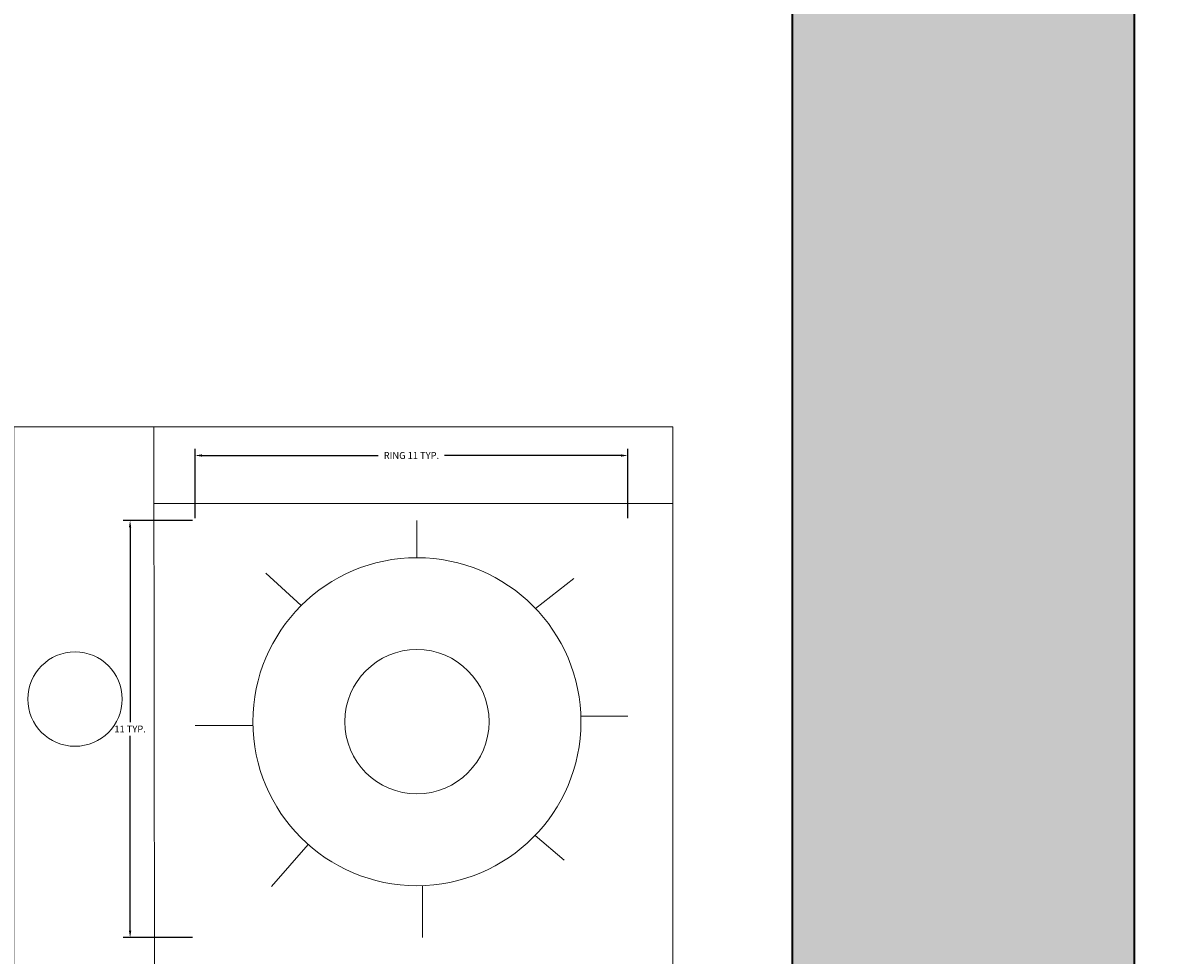
# Model space of a CAD drawing. Units: inches. Extents: x 1568 to 2529, y 2149 to 2897.
# Tile 7 of 16: x 1944 to 1974, y 2386 to 2410. Entities that reach past the tile are written whole.
import ezdxf

# ---------------------------------------------------------------- set-up
doc = ezdxf.new("R2010")
doc.units = ezdxf.units.IN
for name, color, linetype, lineweight in [('A-ANNO-DIMS', 2, 'Continuous', 18), ('A-EQPM', 8, 'Continuous', 18), ('A-WALL-PATT', 172, 'Continuous', 13), ('wall', 7, 'Continuous', 35)]:
    doc.layers.add(name, color=color, linetype=linetype, lineweight=lineweight)
doc.styles.get("Standard").update_dxf_attribs({"font": 'arial.ttf'})
doc.dimstyles.get("Standard").update_dxf_attribs({"dimtxt": 0.18, "dimasz": 0.18, "dimexe": 0.18, "dimexo": 0.0625, "dimgap": 0.09, "dimtad": 0, "dimtih": 1, "dimtoh": 1, "dimdec": 4, "dimzin": 0, "dimdsep": 46, "dimtxsty": 'Standard', "dimcen": 0.09, "dimadec": 0, "dimazin": 0, "dimtfac": 1, "dimtdec": 4, "dimtofl": 0, "dimtmove": 0, "dimatfit": 3, "dimfxl": 1, "dimtolj": 1, "dimtzin": 0, "dimarcsym": 0})

# ---------------------------------------------------------------- blocks, each defined once
blk = doc.blocks.new('COOKTOP-BURNER')
for p, q in [((0.001, 4.315), (0.001, 5.296)), ((-3.048, 3.054), (-3.977, 3.91)), ((3.12, 2.981), (4.125, 3.765)), ((4.312, 0.148), (5.549, 0.148)), ((-4.314, -0.098), (-5.839, -0.098)), ((3.11, -2.99), (3.87, -3.639)), ((-2.86, -3.23), (-3.831, -4.332)), ((0.143, -4.312), (0.143, -5.681))]:
    blk.add_line(p, q)
for radius in [4.315, 1.899]:
    blk.add_circle((0, 0), radius)
blk = doc.blocks.new('*D25')
at = {"layer": 'A-ANNO-DIMS', "color": 0, "lineweight": -2, "transparency": 16777216}
for p, q in [((1948.831, 2397.253), (1948.831, 2399.078)), ((1949.011, 2398.898), (1953.652, 2398.898)), ((1960.039, 2398.898), (1955.397, 2398.898)), ((1960.219, 2397.253), (1960.219, 2399.078))]:
    blk.add_line(p, q, dxfattribs=at)
at = {"layer": 'A-ANNO-DIMS', "color": 0, "transparency": 16777216}
for points in [[(1949.011, 2398.928), (1949.011, 2398.868), (1948.831, 2398.898)], [(1960.039, 2398.928), (1960.039, 2398.868), (1960.219, 2398.898)]]:
    blk.add_solid(points, dxfattribs=at)
at = {"layer": 'Defpoints', "color": 0, "transparency": 16777216}
for p in [(1960.219, 2398.898), (1948.831, 2397.19), (1960.219, 2397.19)]:
    blk.add_point(p, dxfattribs=at)
at = {"layer": 'A-ANNO-DIMS', "color": 0, "transparency": 16777216, "insert": (1954.525, 2398.898), "char_height": 0.18, "attachment_point": 5}
blk.add_mtext('\\A1;RING 11 TYP.', dxfattribs=at)
blk = doc.blocks.new('*D26')
at = {"layer": 'A-ANNO-DIMS', "color": 0, "lineweight": -2, "transparency": 16777216}
for p, q in [((1948.768, 2397.19), (1946.942, 2397.19)), ((1947.122, 2397.01), (1947.122, 2391.882)), ((1947.122, 2386.393), (1947.122, 2391.521)), ((1948.768, 2386.213), (1946.942, 2386.213))]:
    blk.add_line(p, q, dxfattribs=at)
at = {"layer": 'A-ANNO-DIMS', "color": 0, "transparency": 16777216}
for points in [[(1947.092, 2397.01), (1947.152, 2397.01), (1947.122, 2397.19)], [(1947.092, 2386.393), (1947.152, 2386.393), (1947.122, 2386.213)]]:
    blk.add_solid(points, dxfattribs=at)
at = {"layer": 'Defpoints', "color": 0, "transparency": 16777216}
for p in [(1947.122, 2397.19), (1948.831, 2397.19), (1948.831, 2386.213)]:
    blk.add_point(p, dxfattribs=at)
at = {"layer": 'A-ANNO-DIMS', "color": 0, "transparency": 16777216, "insert": (1947.122, 2391.701), "char_height": 0.18, "attachment_point": 5}
blk.add_mtext('\\A1;11 TYP.', dxfattribs=at)
blk = doc.blocks.new('*D28')
at = {"layer": 'A-ANNO-DIMS', "color": 0, "lineweight": -2, "transparency": 16777216}
for p, q in [((1973.643, 2801.532), (2009.61, 2801.532)), ((2009.43, 2801.352), (2009.43, 2501.714)), ((2009.43, 2201.712), (2009.43, 2501.35)), ((1973.613, 2201.532), (2009.61, 2201.532))]:
    blk.add_line(p, q, dxfattribs=at)
at = {"layer": 'A-ANNO-DIMS', "color": 0, "transparency": 16777216}
for points in [[(2009.4, 2801.352), (2009.46, 2801.352), (2009.43, 2801.532)], [(2009.4, 2201.712), (2009.46, 2201.712), (2009.43, 2201.532)]]:
    blk.add_solid(points, dxfattribs=at)
at = {"layer": 'Defpoints', "color": 0, "transparency": 16777216}
for p in [(1973.58, 2801.532), (2009.43, 2801.532), (1973.551, 2201.532)]:
    blk.add_point(p, dxfattribs=at)
at = {"layer": 'A-ANNO-DIMS', "color": 0, "transparency": 16777216, "insert": (2009.43, 2501.532), "char_height": 0.18, "attachment_point": 5}
blk.add_mtext('\\A1;600', dxfattribs=at)
blk = doc.blocks.new('*D32')
at = {"layer": 'A-ANNO-DIMS', "color": 0, "lineweight": -2, "transparency": 16777216}
for p, q in [((1964.551, 2792.469), (1964.551, 2165.502)), ((1904.551, 2753.401), (1904.551, 2165.502)), ((1904.731, 2165.682), (1934.332, 2165.682)), ((1964.371, 2165.682), (1934.77, 2165.682))]:
    blk.add_line(p, q, dxfattribs=at)
at = {"layer": 'A-ANNO-DIMS', "color": 0, "transparency": 16777216}
for points in [[(1904.731, 2165.712), (1904.731, 2165.652), (1904.551, 2165.682)], [(1964.371, 2165.712), (1964.371, 2165.652), (1964.551, 2165.682)]]:
    blk.add_solid(points, dxfattribs=at)
at = {"layer": 'Defpoints', "color": 0, "transparency": 16777216}
for p in [(1964.551, 2792.532), (1904.551, 2753.463), (1964.551, 2165.682)]:
    blk.add_point(p, dxfattribs=at)
at = {"layer": 'A-ANNO-DIMS', "color": 0, "transparency": 16777216, "insert": (1934.551, 2165.682), "char_height": 0.18, "attachment_point": 5}
blk.add_mtext('\\A1;60', dxfattribs=at)

msp = doc.modelspace()

# ---------------------------------------------------------------- hatches: boundary and pattern name
at = {"layer": 'A-WALL-PATT'}
h = msp.add_hatch(color=256, dxfattribs=at)
h.dxf.hatch_style = 1
h.paths.add_polyline_path([(1738.1593, 2801.532), (1634.4841, 2801.532), (1634.4841, 2792.532), (1738.1593, 2792.532)])
h.paths.add_polyline_path([(1812.4114, 2801.532), (1759.0925, 2801.532), (1759.0925, 2792.532), (1812.4114, 2792.532)])
h.paths.add_polyline_path([(1952.647, 2801.532), (1848.4114, 2801.532), (1848.4114, 2792.532), (1952.647, 2792.532)])
h.paths.add_polyline_path([(1973.5509, 2792.532), (1964.5509, 2792.532), (1964.5509, 2699.1671), (1973.5509, 2699.1671)])
h.paths.add_polyline_path([(1973.5509, 2663.1671), (1964.5509, 2663.1671), (1964.5509, 2630.5978), (1973.5509, 2630.5978)])
h.paths.add_polyline_path([(1973.5509, 2609.6646), (1964.5509, 2609.6646), (1964.5509, 2572.3679), (1973.5509, 2572.3679)])
h.paths.add_polyline_path([(1622.5509, 2753.3576), (1622.3864, 2753.3576), (1613.5509, 2753.3576), (1613.5509, 2705.9172), (1622.5509, 2705.9172)])
h.paths.add_polyline_path([(1622.5509, 2669.9172), (1613.5509, 2669.9172), (1613.5509, 2624.532), (1622.5509, 2624.532)])
h.paths.add_polyline_path([(1759.0509, 2757.9833), (1754.5509, 2757.9833), (1754.5509, 2744.532), (1622.5509, 2744.532), (1622.5509, 2740.032), (1754.5509, 2740.032), (1754.5509, 2730.8156), (1759.0509, 2730.8156), (1759.0509, 2740.032)])
h.paths.add_polyline_path([(1759.0509, 2690.8156), (1754.5509, 2690.8156), (1754.5509, 2624.532), (1759.0509, 2624.532)])
h.paths.add_polyline_path([(1738.1177, 2620.032), (1634.4841, 2620.032), (1634.4841, 2615.532), (1738.1177, 2615.532)])
h.paths.add_polyline_path([(1622.5509, 2615.532), (1613.5509, 2615.532), (1613.5509, 2564.2764), (1622.5509, 2564.2764)])
h.paths.add_polyline_path([(1759.0509, 2411.2271), (1754.5509, 2411.2271), (1754.5509, 2339.532), (1759.0509, 2339.532)])
h.paths.add_polyline_path([(1759.0509, 2464.032), (1734.3925, 2464.032), (1622.5509, 2464.032), (1622.5509, 2459.532), (1736.5509, 2459.532), (1754.5509, 2459.532), (1754.5509, 2451.2271), (1759.0509, 2451.2271)])
h.paths.add_polyline_path([(1844.5509, 2471.532), (1858.1805, 2471.532), (1858.1805, 2476.032), (1844.5509, 2476.032), (1844.5509, 2510.0763), (1840.0509, 2510.0763), (1840.0509, 2476.032), (1840.0509, 2339.532), (1844.5509, 2339.532)])
h.paths.add_polyline_path([(1844.5509, 2596.032), (1964.5509, 2596.032), (1964.5509, 2600.532), (1840.0509, 2600.532), (1840.0509, 2570.0763), (1844.5509, 2570.0763)])
h.paths.add_polyline_path([(1964.5509, 2476.032), (1894.1805, 2476.032), (1894.1805, 2471.532), (1964.5509, 2471.532)])
h.paths.add_polyline_path([(1622.5509, 2528.2764), (1613.5509, 2528.2764), (1613.5509, 2436.512), (1622.5509, 2436.512)])
h.paths.add_polyline_path([(1622.5509, 2400.512), (1613.5509, 2400.512), (1613.5509, 2339.532), (1622.5509, 2339.532)])
h.paths.add_polyline_path([(1738.9144, 2339.532), (1634.4841, 2339.532), (1634.4841, 2330.532), (1738.9144, 2330.532)])
h.paths.add_polyline_path([(1792.463, 2336.532, -0.0187698), (1792.5756, 2339.532), (1783.8928, 2339.532), (1783.8928, 2330.532), (1792.463, 2330.532)])
h.paths.add_polyline_path([(1952.6177, 2339.532), (1885.2912, 2339.532), (1885.2912, 2330.532), (1952.6177, 2330.532)])
h.paths.add_polyline_path([(1973.5509, 2422.371), (1964.5509, 2422.371), (1964.5509, 2395.032), (1964.5509, 2387.286), (1964.5509, 2339.532), (1973.5509, 2339.532)])
h.paths.add_polyline_path([(1973.5509, 2536.3679), (1964.5509, 2536.3679), (1964.5509, 2476.032), (1964.5509, 2458.371), (1973.5509, 2458.371)])

# ---------------------------------------------------------------- linework, layer by layer
at = {"layer": 'A-EQPM'}
for p, q in [((1947.7496, 2399.6535), (1947.7862, 2365.7088)), ((1947.7518, 2397.6386), (1961.4053, 2397.6386))]:
    msp.add_line(p, q, dxfattribs=at)
msp.add_lwpolyline([(1944.063, 2365.7088), (1961.4053, 2365.7088), (1961.4053, 2399.6535), (1944.063, 2399.6535)], close=True, dxfattribs=at)
msp.add_circle((1945.6729, 2392.4888), 1.2412, dxfattribs=at)
at = {"layer": 'wall'}
msp.add_line((1964.5509, 2387.286), (1964.5509, 2414.1822), dxfattribs=at)
msp.add_lwpolyline([(1613.5509, 2201.532), (1973.5509, 2201.532), (1973.5509, 2801.532), (1613.5509, 2801.532)], close=True, dxfattribs=at)
for points in [[(1964.5509, 2395.032), (1964.5509, 2792.532), (1622.5509, 2792.532), (1622.5509, 2624.532)], [(1964.5509, 2339.532), (1964.5509, 2390.532)]]:
    msp.add_lwpolyline(points, dxfattribs=at)

# ---------------------------------------------------------------- block references
at = {"layer": 'A-EQPM'}
msp.add_blockref('COOKTOP-BURNER', (1954.6696, 2391.894), dxfattribs=at)

# ---------------------------------------------------------------- dimensions: what is measured, and where the dimension line sits
at = {"layer": 'A-ANNO-DIMS'}
dim = msp.add_linear_dim(base=(2009.4302, 2801.532), p1=(1973.5509, 2201.532), p2=(1973.5802, 2801.532), angle=90, dimstyle='Standard', override={"dimdec": 0, "dimlfac": 1, "dimrnd": 0, "dimzin": 0, "dimdsep": 46, "dimlunit": 2}, dxfattribs=at)
dim.commit()
dim.dimension.update_dxf_attribs({"geometry": '*D28', "text_midpoint": (2009.4302, 2501.532)})
dim = msp.add_linear_dim(base=(1964.5509, 2165.682), p1=(1904.5509, 2753.4635), p2=(1964.5509, 2792.532), dimstyle='Standard', override={"dimdec": 0, "dimlfac": 1, "dimrnd": 0, "dimzin": 0, "dimdsep": 46, "dimlunit": 2}, dxfattribs=at)
dim.commit()
dim.dimension.update_dxf_attribs({"geometry": '*D32', "text_midpoint": (1934.5509, 2165.682)})
dim = msp.add_linear_dim(base=(1960.2186, 2398.8985), p1=(1948.8306, 2397.1903), p2=(1960.2186, 2397.1903), text='RING <> TYP.', dimstyle='Standard', override={"dimdec": 0, "dimlfac": 1, "dimrnd": 0, "dimzin": 0, "dimdsep": 46, "dimlunit": 2}, dxfattribs=at)
dim.commit()
dim.dimension.update_dxf_attribs({"geometry": '*D25', "text_midpoint": (1954.5246, 2398.8985)})
dim = msp.add_linear_dim(base=(1947.1224, 2397.1903), p1=(1948.8306, 2386.2127), p2=(1948.8306, 2397.1903), angle=90, text='<> TYP.', dimstyle='Standard', override={"dimdec": 0, "dimlfac": 1, "dimrnd": 0, "dimzin": 0, "dimdsep": 46, "dimlunit": 2}, dxfattribs=at)
dim.commit()
dim.dimension.update_dxf_attribs({"geometry": '*D26', "text_midpoint": (1947.1224, 2391.7015)})

doc.saveas('drawing.dxf')
